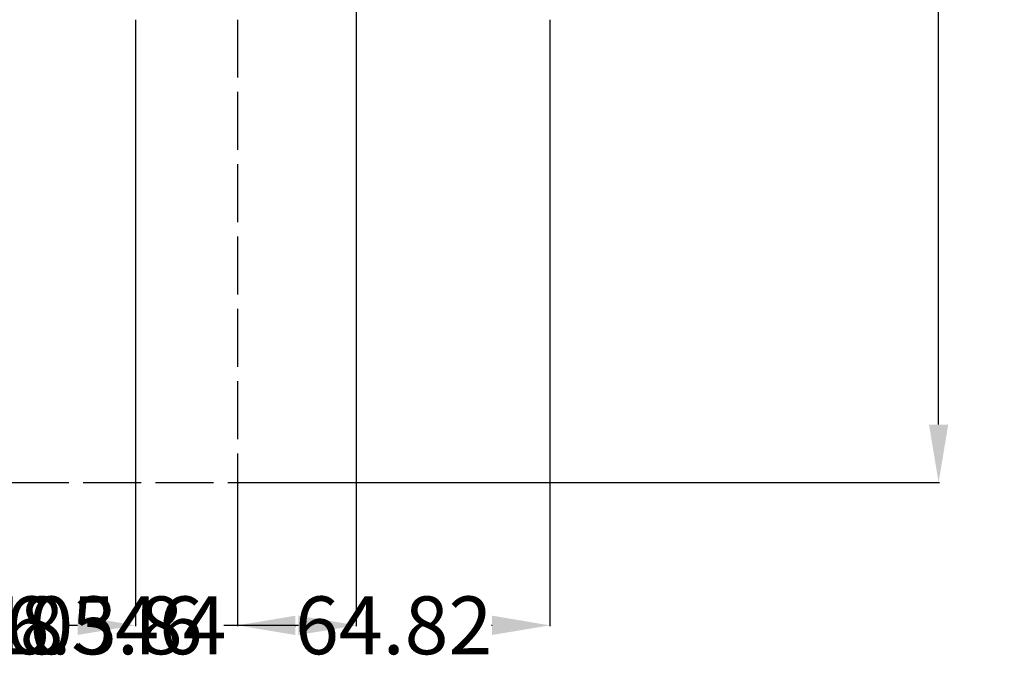
# Model space of a CAD drawing. Units: inches. Extents: x -77 to 516, y -119 to 536.
# Tile 3 of 11: x 264 to 468, y -119 to 15. Entities that reach past the tile are written whole.
import ezdxf

# ---------------------------------------------------------------- set-up
doc = ezdxf.new("R2010")
doc.units = ezdxf.units.IN
doc.header["$MEASUREMENT"] = 0
doc.linetypes.add('ACAD_ISO02W100', pattern=[15, 12, -3])
doc.layers.add('A-ANNO-DIMS', color=2, linetype='Continuous', lineweight=18)
doc.layers.add('A-FLOR-PRCH', color=40, linetype='ACAD_ISO02W100', lineweight=25)
doc.styles.get("Standard").update_dxf_attribs({"font": 'arial.ttf'})
doc.dimstyles.get("Standard").update_dxf_attribs({"dimtxt": 12, "dimasz": 12, "dimexe": 0.18, "dimexo": 0.0625, "dimgap": 0.09, "dimtad": 0, "dimtih": 1, "dimtoh": 1, "dimdec": 1, "dimzin": 0, "dimdsep": 46, "dimlunit": 4, "dimtxsty": 'Standard', "dimcen": 0.09, "dimadec": 0, "dimazin": 0, "dimtfac": 1, "dimtdec": 1, "dimtofl": 0, "dimtmove": 0, "dimatfit": 3, "dimfxl": 1, "dimtolj": 1, "dimtzin": 0, "dimarcsym": 0})

# ---------------------------------------------------------------- blocks, each defined once
blk = doc.blocks.new('*D37')
at = {"layer": 'A-ANNO-DIMS', "color": 0, "lineweight": -2, "transparency": 16777216}
for p, q in [((373.81, 494.59), (454.58, 494.59)), ((454.4, 482.59), (454.4, 212.81)), ((454.4, -69.41), (454.4, 200.37)), ((309, -81.41), (454.58, -81.41))]:
    blk.add_line(p, q, dxfattribs=at)
at = {"layer": 'A-ANNO-DIMS', "color": 0, "transparency": 16777216}
for points in [[(452.4, 482.59), (456.4, 482.59), (454.4, 494.59)], [(452.4, -69.41), (456.4, -69.41), (454.4, -81.41)]]:
    blk.add_solid(points, dxfattribs=at)
at = {"layer": 'Defpoints', "color": 0, "transparency": 16777216}
for p in [(373.75, 494.59), (454.4, 494.59), (308.93, -81.41)]:
    blk.add_point(p, dxfattribs=at)
at = {"layer": 'A-ANNO-DIMS', "color": 0, "transparency": 16777216, "insert": (454.4, 206.59), "char_height": 12, "attachment_point": 5}
blk.add_mtext('\\A1;576', dxfattribs=at)
blk = doc.blocks.new('*D38')
at = {"layer": 'A-ANNO-DIMS', "color": 0, "lineweight": -2, "transparency": 16777216}
for p, q in [((373.75, 14.53), (373.75, -111.24)), ((308.93, -81.47), (308.93, -111.24)), ((320.93, -111.06), (321.03, -111.06)), ((361.75, -111.06), (361.65, -111.06))]:
    blk.add_line(p, q, dxfattribs=at)
at = {"layer": 'A-ANNO-DIMS', "color": 0, "transparency": 16777216}
for points in [[(320.93, -109.06), (320.93, -113.06), (308.93, -111.06)], [(361.75, -109.06), (361.75, -113.06), (373.75, -111.06)]]:
    blk.add_solid(points, dxfattribs=at)
at = {"layer": 'Defpoints', "color": 0, "transparency": 16777216}
for p in [(373.75, 14.59), (308.93, -81.41), (373.75, -111.06)]:
    blk.add_point(p, dxfattribs=at)
at = {"layer": 'A-ANNO-DIMS', "color": 0, "transparency": 16777216, "insert": (341.34, -111.06), "char_height": 12, "attachment_point": 5}
blk.add_mtext('\\A1;64.82', dxfattribs=at)
blk = doc.blocks.new('*D41')
at = {"layer": 'A-ANNO-DIMS', "color": 0, "lineweight": -2, "transparency": 16777216}
for p, q in [((229.75, 485.53), (229.75, -111.24)), ((333.59, 485.53), (333.59, -111.24)), ((241.75, -111.06), (257.26, -111.06)), ((321.59, -111.06), (306.08, -111.06))]:
    blk.add_line(p, q, dxfattribs=at)
at = {"layer": 'A-ANNO-DIMS', "color": 0, "transparency": 16777216}
for points in [[(241.75, -109.06), (241.75, -113.06), (229.75, -111.06)], [(321.59, -109.06), (321.59, -113.06), (333.59, -111.06)]]:
    blk.add_solid(points, dxfattribs=at)
at = {"layer": 'Defpoints', "color": 0, "transparency": 16777216}
for p in [(229.75, 485.59), (333.59, 485.59), (333.59, -111.06)]:
    blk.add_point(p, dxfattribs=at)
at = {"layer": 'A-ANNO-DIMS', "color": 0, "transparency": 16777216, "insert": (281.67, -111.06), "char_height": 12, "attachment_point": 5}
blk.add_mtext('\\A1;103.84', dxfattribs=at)
blk = doc.blocks.new('*D51')
at = {"layer": 'A-ANNO-DIMS', "color": 0, "lineweight": -2, "transparency": 16777216}
for p, q in [((203.2, 14.53), (203.2, -111.24)), ((239.75, 14.53), (239.75, -111.24)), ((215.2, -111.06), (227.75, -111.06)), ((239.75, -111.06), (251.75, -111.06))]:
    blk.add_line(p, q, dxfattribs=at)
at = {"layer": 'A-ANNO-DIMS', "color": 0, "transparency": 16777216}
for points in [[(215.2, -109.06), (215.2, -113.06), (203.2, -111.06)], [(227.75, -109.06), (227.75, -113.06), (239.75, -111.06)]]:
    blk.add_solid(points, dxfattribs=at)
at = {"layer": 'Defpoints', "color": 0, "transparency": 16777216}
for p in [(203.2, 14.59), (239.75, 14.59), (239.75, -111.06)]:
    blk.add_point(p, dxfattribs=at)
at = {"layer": 'A-ANNO-DIMS', "color": 0, "transparency": 16777216, "insert": (276.74, -111.06), "char_height": 12, "attachment_point": 5}
blk.add_mtext('\\A1;36.546', dxfattribs=at)
blk = doc.blocks.new('*D52')
at = {"layer": 'A-ANNO-DIMS', "color": 0, "lineweight": -2, "transparency": 16777216}
for p, q in [((239.75, 14.53), (239.75, -111.24)), ((287.75, 14.53), (287.75, -111.24)), ((251.75, -111.06), (254.81, -111.06)), ((275.75, -111.06), (272.69, -111.06))]:
    blk.add_line(p, q, dxfattribs=at)
at = {"layer": 'A-ANNO-DIMS', "color": 0, "transparency": 16777216}
for points in [[(251.75, -109.06), (251.75, -113.06), (239.75, -111.06)], [(275.75, -109.06), (275.75, -113.06), (287.75, -111.06)]]:
    blk.add_solid(points, dxfattribs=at)
at = {"layer": 'Defpoints', "color": 0, "transparency": 16777216}
for p in [(239.75, 14.59), (287.75, 14.59), (287.75, -111.06)]:
    blk.add_point(p, dxfattribs=at)
at = {"layer": 'A-ANNO-DIMS', "color": 0, "transparency": 16777216, "insert": (263.75, -111.06), "char_height": 12, "attachment_point": 5}
blk.add_mtext('\\A1;48', dxfattribs=at)

msp = doc.modelspace()

# ---------------------------------------------------------------- linework, layer by layer
at = {"layer": 'A-FLOR-PRCH'}
msp.add_line((308.9336, 14.5884), (308.9336, -81.4116), dxfattribs=at)
msp.add_lwpolyline([(156.9336, -81.4116), (308.9336, -81.4116)], dxfattribs=at)

# ---------------------------------------------------------------- dimensions: what is measured, and where the dimension line sits
at = {"layer": 'A-ANNO-DIMS'}
dim = msp.add_linear_dim(base=(454.4001, 494.5884), p1=(308.9336, -81.4116), p2=(373.7501, 494.5884), angle=90, dimstyle='Standard', override={"dimdec": 0, "dimlfac": 1, "dimrnd": 0, "dimzin": 0, "dimdsep": 46, "dimlunit": 2}, dxfattribs=at)
dim.commit()
dim.dimension.update_dxf_attribs({"geometry": '*D37', "text_midpoint": (454.4001, 206.5884)})
for base, p1, p2, override, picture, middle in [((333.5885, -111.0616), (229.7501, 485.5884), (333.5885, 485.5884), {"dimdec": 2, "dimlfac": 1, "dimrnd": 0, "dimzin": 0, "dimdsep": 46, "dimlunit": 2}, '*D41', (281.6693, -111.0616)), ((239.7501, -111.0616), (203.2037, 14.5884), (239.7501, 14.5884), {"dimdec": 3, "dimlfac": 1, "dimrnd": 0, "dimzin": 0, "dimdsep": 46, "dimlunit": 2}, '*D51', (276.7405, -111.0616)), ((287.7501, -111.0616), (239.7501, 14.5884), (287.7501, 14.5884), {"dimdec": 0, "dimlfac": 1, "dimrnd": 0, "dimzin": 0, "dimdsep": 46, "dimlunit": 2}, '*D52', (263.7501, -111.0616)), ((373.7501, -111.0616), (308.9336, -81.4116), (373.7501, 14.5884), {"dimdec": 2, "dimlfac": 1, "dimrnd": 0, "dimzin": 0, "dimdsep": 46, "dimlunit": 2}, '*D38', (341.3418, -111.0616))]:
    dim = msp.add_linear_dim(base=base, p1=p1, p2=p2, dimstyle='Standard', override=override, dxfattribs=at)
    dim.commit()
    dim.dimension.update_dxf_attribs({"geometry": picture, "text_midpoint": middle})

doc.saveas('drawing.dxf')
